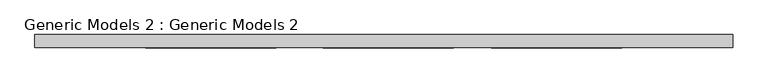
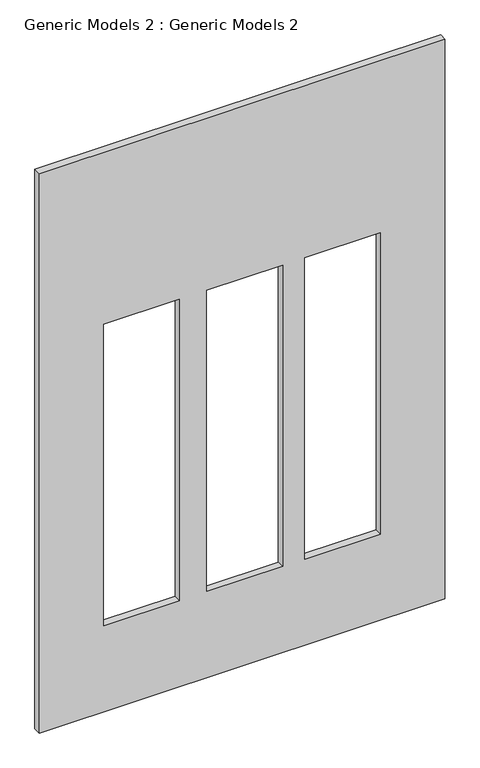
"""IFC4 building model written with IfcOpenShell, lengths in millimetres: proxy geometry, Generic Models 2 : Generic Models 2."""

from ifc_helpers import new_model, si_unit, frame, origin, place, context, project, spatial, polyline, outline, extrude, source, transform, mapped, element, save


def generic_models_2_generic_models_2_65ba8ebd(model_context):
    return source(origin(), model_context, "Body", "SweptSolid", [
        extrude(outline(polyline([(7010.4, -8399.3906521), (3048.0, -8399.3906521), (3048.0, -5681.5906521), (7010.4, -5681.5906521), (7010.4, -8399.3906521)]), holes=[polyline([(5791.2, -7460.2171142), (3657.6, -7460.2171142), (3657.6, -7968.2171142), (5791.2, -7968.2171142), (5791.2, -7460.2171142)]), polyline([(5791.2, -6768.0671142), (3657.6, -6768.0671142), (3657.6, -7276.0671142), (5791.2, -7276.0671142), (5791.2, -6768.0671142)]), polyline([(5791.2, -6114.0171142), (3657.6, -6114.0171142), (3657.6, -6622.0171142), (5791.2, -6622.0171142), (5791.2, -6114.0171142)])]), frame((0.0, -12127.0453012, 0.0), z_axis=(0.0, 1.0, 0.0), x_axis=(0.0, 0.0, 1.0)), (0.0, 0.0, 1.0), 50.8),
    ])


if __name__ == "__main__":
    model = new_model("IFC4")
    model_context = context("Model", 3, world=origin())
    ifc_project = project(units=[si_unit("LENGTHUNIT", "METRE", prefix="MILLI")], contexts=[model_context])
    site = spatial("IfcSite", under=ifc_project)
    building = spatial("IfcBuilding", under=site)
    placement = place(None, origin())
    generic_models_2_generic_models_2_shape = generic_models_2_generic_models_2_65ba8ebd(model_context)
    element("IfcBuildingElementProxy", 1, Name="Generic Models 2 : Generic Models 2", ObjectType="Generic Models 2 : Generic Models 2", at=placement, inside=building, context=model_context, shape_type="MappedRepresentation", body=[
        mapped(generic_models_2_generic_models_2_shape, transform((0.0, 0.0, 0.0), x_axis=(1.0, 0.0, 0.0), y_axis=(0.0, 1.0, 0.0), z_axis=(0.0, 0.0, 1.0))),
    ])
    save(model, "model.ifc")

# Revit data of these elements
# Element 1 (IfcBuildingElementProxy, "Generic Models 2 : Generic Models 2")
#   Materials on its faces: "GREY COLOUR FRAME"
# Materials
#   "GREY COLOUR FRAME": class "Generic", colour RGB 120 120 120, transparency 0, Cost = 0
